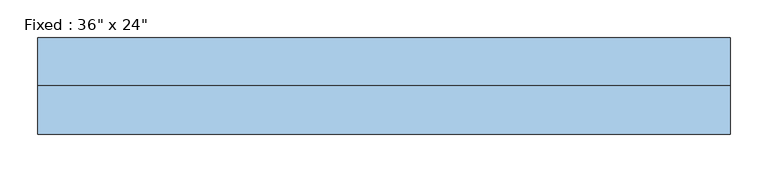
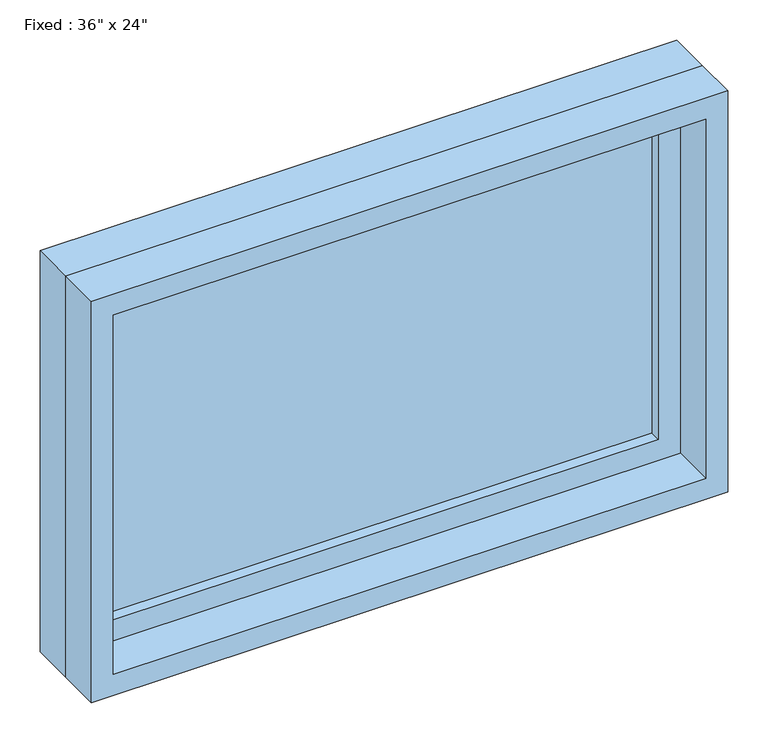
"""IFC4 building model written with IfcOpenShell, lengths in millimetres: window geometry."""

from ifc_helpers import new_model, si_unit, frame, origin, place, context, project, spatial, polyline, outline, extrude, source, transform, mapped, element, save


def window_12349545(model_context):
    return source(origin(), model_context, "Body", "SweptSolid", [
        extrude(outline(polyline([(355.6, 15.875), (-431.8, 15.875), (-431.8, 28.575), (355.6, 28.575), (355.6, 15.875)])), frame((0.0, 0.0, 2197.1), z_axis=(0.0, 0.0, 1.0), x_axis=(1.0, 0.0, 0.0)), (0.0, 0.0, 1.0), 482.6),
        extrude(outline(polyline([(2724.15, -476.25), (2152.65, -476.25), (2152.65, 400.05), (2724.15, 400.05), (2724.15, -476.25)]), holes=[polyline([(2679.7, -431.8), (2679.7, 355.6), (2197.1, 355.6), (2197.1, -431.8), (2679.7, -431.8)])]), frame((0.0, 0.0, 0.0), z_axis=(0.0, 1.0, 0.0), x_axis=(0.0, 0.0, 1.0)), (0.0, 0.0, 1.0), 44.45),
        extrude(outline(polyline([(2743.2, -495.3), (2133.6, -495.3), (2133.6, 419.1), (2743.2, 419.1), (2743.2, -495.3)]), holes=[polyline([(2711.45, -463.55), (2711.45, 387.35), (2165.35, 387.35), (2165.35, -463.55), (2711.45, -463.55)])]), frame((0.0, -63.5, 0.0), z_axis=(0.0, 1.0, 0.0), x_axis=(0.0, 0.0, 1.0)), (0.0, 0.0, 1.0), 63.5),
        extrude(outline(polyline([(2743.2, 419.1), (2743.2, -495.3), (2133.6, -495.3), (2133.6, 419.1), (2743.2, 419.1)]), holes=[polyline([(2724.15, 400.05), (2152.65, 400.05), (2152.65, -476.25), (2724.15, -476.25), (2724.15, 400.05)])]), frame((0.0, 0.0, 0.0), z_axis=(0.0, 1.0, 0.0), x_axis=(0.0, 0.0, 1.0)), (0.0, 0.0, 1.0), 63.5),
    ])


if __name__ == "__main__":
    model = new_model("IFC4")
    model_context = context("Model", 3, world=origin())
    ifc_project = project(units=[si_unit("LENGTHUNIT", "METRE", prefix="MILLI")], contexts=[model_context])
    site = spatial("IfcSite", under=ifc_project)
    building = spatial("IfcBuilding", under=site)
    placement = place(None, origin())
    window_shape = window_12349545(model_context)
    element("IfcWindow", 1, ObjectType="Fixed : 36\" x 24\"", at=placement, inside=building, context=model_context, shape_type="MappedRepresentation", body=[
        mapped(window_shape, transform((0.0, 0.0, 0.0), x_axis=(1.0, 0.0, 0.0), y_axis=(0.0, 1.0, 0.0), z_axis=(0.0, 0.0, 1.0))),
    ])
    save(model, "model.ifc")

# Revit data of these elements
# Type "Fixed : 36\" x 24\""
#   Type Mark = "8"
#   Construction Type Id = "GSP4R"
#   Assembly Code = "B2020100"
#   Analytic Construction = "1/8 in Pilkington single glazing"
#   Visual Light Transmittance = 0.9
#   Solar Heat Gain Coefficient = 0.78
#   Heat Transfer Coefficient (U) = 0.6496 BTU/(h·ft²·°F)
#   Height = 2' - 0"
#   Default Sill Height = 7' - 0"
#   Width = 3' - 0"
#   Window Inset = 0' - 0 3/4"
#   Define Thermal Properties by = 1
#   Define Thermal Properties by = 1
#   Glass Pane Material = Glass
#   Sash Material = Sash
#   Wall Closure = (empty or 0)
# Element 1 (IfcWindow, "Fixed : 36\" x 24\"")
#   Materials on its faces: "Sash", "Glass"
# Materials
#   "Glass": class "Glass", colour RGB 0 128 192, transparency 0.75, Description = "Soda Lime Glass", Cost = 0
#   "Sash": class "Wood", colour RGB 224 178 126, transparency 0, Cost = 0
